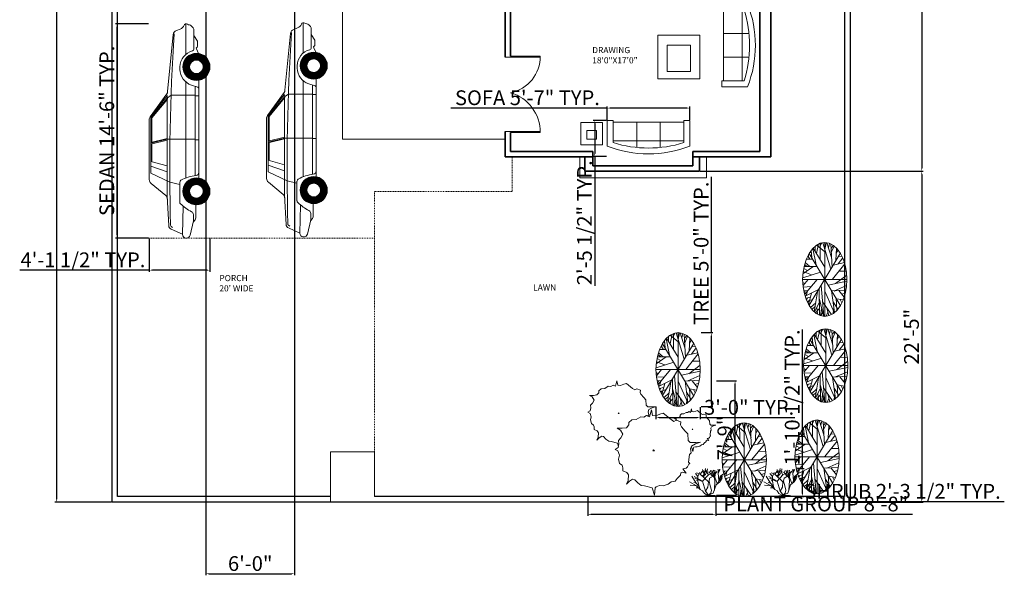
# Model space of a CAD drawing. Units: inches. Extents: x 2562 to 3392, y 1021 to 2243.
# Tile 1 of 6: x 2562 to 3362, y 1021 to 1472. Entities that reach past the tile are written whole.
import ezdxf

# ---------------------------------------------------------------- set-up
doc = ezdxf.new("R2010")
doc.units = ezdxf.units.IN
doc.linetypes.add('JIS_02_0.7', pattern=[1.35, 0.75, -0.6])
for name, color, linetype, lineweight in [('A-ANNO-DIMS', 2, 'Continuous', 18), ('A-ANNO-SYMB', 7, 'Continuous', 13), ('A-AREA-IDEN', 7, 'Continuous', 18), ('A-DOOR', 4, 'Continuous', 18), ('A-FLOR-STRS', 7, 'Continuous', 18), ('A-FURN', 8, 'Continuous', 18), ('A-WALL', 7, 'Continuous', 35), ('C-PKNG-VEHS', 8, 'Continuous', 13), ('C-PROP', 7, 'Continuous', 30), ('L-HRDS', 8, 'Continuous', 18), ('L-HRDS-HIDN', 8, 'JIS_02_0.7', 13), ('L-PLNT', 94, 'Continuous', 13)]:
    doc.layers.add(name, color=color, linetype=linetype, lineweight=lineweight)
doc.styles.get("Standard").update_dxf_attribs({"font": 'arial.ttf'})
doc.dimstyles.new('ISO-25', dxfattribs={"dimtxt": 12, "dimasz": 2.5, "dimexe": 1.25, "dimexo": 0.625, "dimtad": 1, "dimdec": 1, "dimlunit": 3, "dimtxsty": 'Standard', "dimcen": 2.5, "dimadec": 0, "dimazin": 0, "dimtfac": 1, "dimtdec": 1, "dimtmove": 0, "dimatfit": 3, "dimfxl": 1, "dimarcsym": 0})

# ---------------------------------------------------------------- blocks, each defined once
blk = doc.blocks.new('Sofa - Roundback 7 ft.')
for p, q in [((-12.00002, -32.4421), (-12.00003, -6.5971)), ((11.99997, -32.4421), (11.99998, -6.5971)), ((-36.000027, -34), (-36.000027, -11.4696)), ((-35.999844, -13.3819), (35.9998, -13.3819)), ((35.99998, -34), (35.99998, -11.4696)), ((-36.000027, -32.4421), (35.99998, -32.4421))]:
    blk.add_line(p, q)
for points in [[(-36.000027, -34), (-42.000027, -34), (-42.000027, -8)], [(41.99998, -8), (41.99998, -34), (35.99998, -34)]]:
    blk.add_lwpolyline(points)
for centre, radius, start, end in [((0, -114.25), 114.25, 68.43141, 111.5686), ((-0.00001, -127.1968), 121.1968, 72.72033, 107.2797)]:
    blk.add_arc(centre, radius, start, end)
blk = doc.blocks.new('Tree - deciduous plan')
for p, q in [((-32.6092, 50.4264), (-23.2782, 23.5674)), ((-31.2008, 51.1035), (-0.2149, 20.1818)), ((-26.4472, 46.5894), (-26.2712, 53.8116)), ((-22.0458, 42.0753), (-16.5881, 57.6486)), ((-21.1656, 55.8436), (-0.0388, 45.0094)), ((-12.5388, 54.9406), (-7.9613, 59.4546)), ((-12.3627, 32.1443), (-12.5388, 58.7776)), ((-5.3205, 59.6806), (16.5105, 16.7963)), ((2.426, 54.9406), (-1.4472, 59.9056)), ((0, 59.9996), (0, -60)), ((0.4894, 48.6208), (3.6584, 59.6806)), ((18.2711, 35.5298), (5.419, 59.6806)), ((9.8203, 51.5549), (12.8133, 58.5516)), ((19.6795, 19.5047), (16.3344, 57.6486)), ((17.0387, 51.1035), (23.2006, 55.1666)), ((17.7429, 43.6552), (25.4894, 54.2636)), ((31.6513, 50.8778), (30.2429, 30.5643)), ((31.1232, 42.5267), (35.8767, 48.1693)), ((-49.8627, 32.8214), (-32.7853, 32.8214)), ((-45.8134, 38.2383), (-40.5318, 33.0471)), ((-43.8768, 36.4326), (-44.405, 40.2696)), ((42, 42), (-42, -42)), ((42, -42), (-42, 42)), ((-40.1797, 44.558), (-36.4825, 43.2038)), ((-37.0107, 47.0408), (-35.25, 35.5298)), ((36.2288, 25.1474), (48.9049, 35.0784)), ((37.1091, 37.1098), (46.6161, 37.5612)), ((-32.2571, 20.6333), (-59.1937, 9.348)), ((-57.081, 17.9248), (-47.0458, 14.7649)), ((-56.0247, 20.859), (-20.8134, 20.859)), ((-54.7923, 24.4702), (-47.75, 21.0847)), ((-53.2078, 27.4044), (-40.1797, 20.859)), ((54.3626, 25.3731), (20.9119, 0.3198)), ((23.3767, 23.3417), (53.3063, 27.4044)), ((-59.7219, 2.8025), (-12.0106, 12.0565)), ((-58.6656, 12.7336), (-35.9543, 7.5424)), ((-54.6162, -24.7335), (-20.2853, 0.0941)), ((29.3626, -6.6771), (59.4682, 7.091)), ((38.5175, 13.4107), (58.2359, 13.6364)), ((-60, 0), (60, 0)), ((-59.7219, -4.8714), (-54.2641, -6.6771)), ((-45.2853, -0.1316), (-59.0177, -10.0627)), ((-58.4895, -12.3197), (-36.4825, -11.6426)), ((-14.8275, -15.0282), (-14.6515, -57.6865)), ((-10.074, -10.0627), (-2.5036, -59.7178)), ((9.2922, -9.1598), (59.6443, -2.8401)), ((26.3697, -18.4138), (58.9401, -9.8369)), ((-57.081, -18.4138), (-45.2853, -17.9624)), ((-52.6797, -18.188), (-55.4966, -22.0251)), ((-53.2078, -27.442), (-16.7641, -16.6081)), ((-38.9472, -29.0219), (-51.4472, -30.6018)), ((-47.2219, -19.3166), (-50.2148, -26.3135)), ((-46.5177, -30.1504), (-49.5106, -33.536)), ((-35.9543, -22.4765), (-44.0529, -40.5329)), ((-19.9331, -20.2194), (-28.5599, -52.721)), ((-0.0388, -19.0909), (25.8415, -53.8495)), ((18.6232, -18.6394), (26.7218, -53.3981)), ((18.7992, -18.6394), (57.3556, -17.2853)), ((30.419, -30.1504), (32.3556, -50.0125)), ((31.4753, -31.279), (49.6091, -33.3103)), ((38.1654, -18.188), (52.426, -29.0219)), ((45.9119, -24.0564), (55.595, -22.2508)), ((-32.4331, -32.4075), (-48.1021, -35.5674)), ((-43.7008, -34.6645), (-46.6937, -37.373)), ((-24.6867, -37.8244), (-38.7712, -45.7241)), ((-26.2712, -43.9185), (-34.7219, -48.6583)), ((-14.6515, -36.2445), (-27.6797, -52.9467)), ((-14.6515, -47.3041), (-25.0388, -54.3009)), ((-21.5177, -45.4984), (-19.9331, -56.1065)), ((-14.6515, -32.1818), (-3.912, -59.4922)), ((-8.4895, -47.5298), (-11.4825, -58.5893)), ((-6.2008, -36.2445), (17.919, -57.0094)), ((5.9471, -46.6269), (10.5246, -58.5893)), ((22.8485, -36.4702), (35.3485, -48.4326)), ((24.7852, -44.8213), (23.0246, -54.978)), ((41.5105, -32.6332), (46.088, -38.0501)), ((-6.3768, -52.721), (-9.3698, -58.815)), ((8.4119, -53.1724), (3.8344, -59.4922))]:
    blk.add_line(p, q)
blk.add_circle((0, 0), 60)
blk = doc.blocks.new('Shrub - elevation')
for p, q in [((-18.24, 11.04), (-21.755, 16.655)), ((-12.96, 12.48), (-19.68, 16.32)), ((-16.8, 16.32), (-18.72, 18.72)), ((-14.88, 18.24), (-17.76, 19.2)), ((-16.8, 16.32), (-15.36, 19.68)), ((-16.8, 12.48), (-16.8, 16.32)), ((-14.88, 18.24), (-12.96, 20.64)), ((-8.16, 12), (-14.88, 18.24)), ((-13.325, 16.724), (-11.433, 18.289)), ((-12.96, 12.48), (-8.16, 17.76)), ((-12.471, 19.775), (-12.898, 22.044)), ((-11.677, 19.071), (-12.471, 19.775)), ((-11.28, 19.619), (-12.104, 21.184)), ((-12.043, 15.628), (-11.921, 18.836)), ((-11.982, 16.802), (-10.579, 18.054)), ((-11.921, 18.836), (-10.64, 20.401)), ((-11.433, 18.289), (-10.457, 22.749)), ((-10.579, 18.054), (-9.846, 19.697)), ((-8.16, 17.76), (-10.56, 21.6)), ((-9.48, 19.775), (-8.992, 22.592)), ((-7.2, 19.68), (-8.64, 20.16)), ((-8.16, 17.76), (-5.28, 19.2)), ((-7.2, 19.68), (-6.24, 21.12)), ((-4.8, 16.32), (-7.2, 19.68)), ((-7.2, 14.88), (-3.84, 16.8)), ((-5.086, 17.741), (-5.513, 21.34)), ((-5.28, 19.2), (-3.84, 21.6)), ((-3.377, 15.315), (-5.086, 17.819)), ((-2.88, 12.96), (-4.32, 19.68)), ((-3.84, 16.8), (-0.96, 20.64)), ((-3.377, 18.602), (-2.888, 21.575)), ((-2.766, 16.802), (-3.377, 18.602)), ((-2.88, 15.84), (-2.4, 20.16)), ((-0.508, 21.888), (-0.081, 20.558)), ((-0.203, 19.149), (0.102, 21.34)), ((0.346, 13.203), (-0.203, 19.149)), ((-0.142, 19.384), (0.59, 20.401)), ((-0.02, 20.01), (0.896, 21.105)), ((0.041, 20.714), (1.384, 22.044)), ((0.102, 21.34), (0.835, 21.888)), ((0.346, 13.203), (1.323, 16.254)), ((1.323, 16.254), (3.642, 18.289)), ((1.44, 15.36), (2.88, 17.28)), ((2.4, 15.36), (3.36, 16.32)), ((-17.76, 8.64), (-23.663, 11.961)), ((-17.76, 8.64), (-23.128, 9.222)), ((-18.24, 11.04), (-20.16, 11.52)), ((-13.92, 12.48), (-19.2, 14.88)), ((-15.84, 8.16), (-18.24, 11.04)), ((-16.8, 12.48), (-17.76, 12.96)), ((-14.88, 5.76), (-17.76, 8.64)), ((-15.84, 8.16), (-16.8, 12.48)), ((-14.88, 5.76), (-15.84, 8.16)), ((-12.96, 12.48), (-13.92, 12.48)), ((-10.56, 4.32), (-12.96, 12.48)), ((-8.64, 7.68), (-8.16, 12)), ((-7.68, 12.48), (-7.2, 14.88)), ((-6.72, 8.64), (-7.68, 12.48)), ((-5.76, 5.28), (-6.72, 8.64)), ((-4.32, 2.88), (-1.92, 9.6)), ((-3.36, 5.28), (-2.88, 12.96)), ((-0.96, 10.56), (-2.88, 15.84)), ((-1.92, 9.6), (0.96, 12)), ((-0.48, 10.8), (0.346, 13.203)), ((0.96, 12), (1.44, 15.36)), ((0.96, 12), (2.88, 14.88)), ((1.92, 13.44), (2.4, 15.36)), ((-16.32, 7.2), (-18.24, 7.2)), ((-15.84, 0.48), (-17.76, 0)), ((-13.44, 0.48), (-15.84, 0.48)), ((-12.96, 4.8), (-14.88, 5.76)), ((-9.6, 0.96), (-13.44, 0.48)), ((-11.52, 2.4), (-12.96, 4.8)), ((-9.6, 0.96), (-12.96, 0)), ((-8.64, 0.96), (-11.52, 2.4)), ((-10.56, 4.32), (-8.64, 7.68)), ((-8.64, 1.92), (-10.56, 4.32)), ((-9.6, 0.96), (-7.68, 0.96)), ((-8.64, 0.96), (-4.32, 2.88)), ((-8.64, 0.96), (-6.24, 2.88)), ((-8.64, 0.96), (-8.64, 1.92)), ((-8.64, 0.96), (-2.88, 0.96)), ((-7.68, 0.96), (-6.24, 0.48)), ((-6.24, 2.88), (-5.76, 5.28)), ((-6.24, 0.48), (-3.36, 0)), ((-2.88, 0.96), (0, 0))]:
    blk.add_line(p, q)
blk = doc.blocks.new('Clump of Trees or Bushes - plan')
for points in [[(-10.993, 56.487), (-9.228, 58.426), (-10.144, 63.512), (-8.923, 67.033), (-3.43, 69.772), (2.673, 72.119), (-2.82, 71.728), (-10.449, 71.728), (-13.195, 74.075), (-13.806, 83.073), (-16.857, 86.594), (-22.045, 92.071), (-22.961, 94.81), (-22.656, 98.722), (-28.759, 100.678), (-31.811, 99.113), (-35.472, 101.461), (-45.543, 109.676), (-49.815, 108.503), (-55.308, 106.155), (-59.58, 106.938), (-60.801, 113.98), (-63.242, 104.982), (-67.209, 106.938), (-70.872, 104.59), (-74.839, 104.982), (-80.637, 101.461), (-86.435, 101.069), (-90.402, 97.548), (-90.402, 94.419), (-93.454, 90.898), (-98.947, 90.115), (-105.66, 90.115), (-101.083, 87.768), (-98.031, 82.682), (-100.778, 77.596), (-103.829, 74.466), (-103.219, 69.772), (-104.134, 65.077), (-108.102, 62.73), (-104.439, 60.774), (-102.609, 55.297), (-103.829, 50.211), (-102.303, 44.342), (-98.947, 41.995), (-98.031, 38.865), (-98.031, 34.953), (-93.148, 32.606), (-90.707, 29.476), (-91.317, 22.434), (-93.454, 17.348), (-89.487, 21.26), (-85.519, 23.999), (-82.468, 23.216), (-78.806, 19.304), (-74.228, 15.783), (-69.956, 15.392), (-59.886, 12.653), (-58.254, 7.074)], [(59.448, 5.262), (60.936, 4.858), (62.652, -1.011), (63.415, 4.858), (64.178, 5.836), (66.848, 6.814), (69.709, 6.569), (73.905, 7.792), (76.385, 9.748), (79.627, 10.237), (81.153, 12.438), (84.014, 15.127), (84.205, 17.084), (85.158, 17.573), (88.591, 16.839), (85.73, 20.262), (88.591, 20.751), (89.545, 21.974), (90.689, 24.174), (91.452, 24.663), (90.499, 25.886), (91.261, 31.999), (92.596, 33.466), (92.024, 36.645), (92.787, 38.845), (96.22, 40.557), (100.035, 42.024), (96.602, 41.779), (91.834, 41.779), (90.117, 43.246), (89.736, 48.871), (87.828, 51.071), (84.586, 54.494), (84.014, 56.206), (84.205, 58.651), (80.39, 59.873), (78.483, 58.895), (76.194, 60.362), (69.9, 65.497), (67.23, 64.764), (63.797, 63.297), (61.126, 63.786), (60.364, 68.187), (58.838, 62.563), (56.358, 63.786), (54.07, 62.319), (51.59, 62.563), (47.966, 60.362), (44.343, 60.118), (41.863, 57.917), (41.863, 55.961), (39.956, 53.761), (36.523, 53.272), (32.327, 53.272), (35.187, 51.805), (36.641, 49.381)]]:
    blk.add_lwpolyline(points)
for points in [[(-4.577, 66.508), (-7.629, 55.261), (-12.588, 57.706), (-17.166, 54.772), (-22.125, 55.261), (-29.372, 50.86), (-36.62, 50.371), (-41.579, 45.969), (-41.579, 42.057), (-45.393, 37.656), (-52.259, 36.678), (-60.651, 36.678), (-54.93, 33.743), (-51.115, 27.386), (-54.548, 21.029), (-58.363, 17.116), (-57.6, 11.248), (-58.744, 5.38), (-63.703, 2.446), (-59.126, 0), (-56.837, -6.846), (-58.363, -13.203), (-56.455, -20.539), (-52.259, -23.473), (-51.115, -27.385), (-51.115, -32.275), (-45.012, -35.21), (-41.96, -39.122), (-42.723, -47.924), (-45.393, -54.282), (-40.434, -49.391), (-35.475, -45.968), (-31.661, -46.946), (-27.083, -51.837), (-21.362, -56.238), (-16.021, -56.727), (-3.433, -60.15), (0, -71.887), (1.526, -60.15), (3.052, -58.194), (8.392, -56.238), (14.114, -56.727), (22.506, -54.282), (27.465, -50.369), (33.949, -49.391), (37.001, -44.99), (42.723, -39.611), (43.104, -35.699), (45.012, -34.721), (51.878, -36.188), (46.156, -29.341), (51.878, -28.363), (53.785, -25.918), (56.074, -21.517), (57.6, -20.539), (55.692, -18.094), (57.218, -5.868), (59.888, -2.934), (58.744, 3.424), (60.27, 7.825), (67.136, 11.248), (74.765, 14.182), (67.899, 13.693), (58.363, 13.693), (54.93, 16.627), (54.167, 27.875), (50.352, 32.276), (43.867, 39.123), (42.723, 42.546), (43.104, 47.436), (35.475, 49.882), (31.661, 47.925), (27.083, 50.86), (14.495, 61.129), (9.155, 59.662), (2.289, 56.728), (-3.052, 57.706)], [(-58.055, 61.947), (-58.97, 60.774), (-57.139, 60.774)], [(62.08, 35.667), (61.508, 34.933), (62.652, 34.933)], [(-1.144, 1.468), (-2.289, 0), (0, 0)]]:
    blk.add_lwpolyline(points, close=True)
blk = doc.blocks.new('Seam Weld')
for p, q in [((-0.2, -0.099999), (0.2, -0.099999)), ((0.2, -0.2), (-0.2, -0.2))]:
    blk.add_line(p, q)
blk.add_circle((0, -0.15), 0.15)
blk = doc.blocks.new('Car - sedan  side')
for p, q in [((-77.81, 49.34), (-126.58, 49.34)), ((-56.87, 35.13), (-75.48, 48.59)), ((-139.53, 35.99), (-129.64, 47.91)), ((-128.57, 32.64), (-121.22, 48.02)), ((-74.7, 48.02), (-121.22, 48.02)), ((-120.32, 34.67), (-115.67, 48.02)), ((-115.4, 34.67), (-111.74, 48.02)), ((-97.55, 47.3), (-111.94, 47.3)), ((-94.41, 34.67), (-97.73, 48.02)), ((-93.72, 34.67), (-97.04, 48.02)), ((-93.03, 34.67), (-96.34, 48.02)), ((-76.26, 47.3), (-96.16, 47.3)), ((-61.08, 34.66), (-76.26, 47.3)), ((-60.02, 34.65), (-76.07, 48.02)), ((-58.54, 34.93), (-74.99, 48.02)), ((-140.23, 34.67), (-163.88, 33.56)), ((-62.28, 34.67), (-140.23, 34.67)), ((-130.39, 24.63), (-128.57, 32.64)), ((-93.72, 19.62), (-93.72, 34.67)), ((-62.28, 34.67), (-60.02, 34.65)), ((-60.02, 34.65), (-58.54, 34.93)), ((-57.97, 31.61), (-60.02, 34.65)), ((-57.21, 35.38), (-58.54, 34.93)), ((-54.93, 34.4), (-8.75, 29.8)), ((-170.93, 22.32), (-166.81, 31.56)), ((-164.57, 31.6), (-165.48, 30.35)), ((-128.78, 24.63), (-144.79, 24.63)), ((-57.97, 19.62), (-57.97, 31.61)), ((-36.97, 24.38), (-34.94, 24.38)), ((-4.21, 24.18), (-5.42, 27.27)), ((-174, 19.51), (-174, 18.91)), ((-160.12, 13.48), (-171.81, 16.16)), ((-148.26, 21.7), (-171.11, 22.33)), ((-47.2, 19.62), (-125.23, 19.62)), ((-93.72, 12.14), (-93.72, 19.62)), ((-57.97, 12.14), (-57.97, 19.62)), ((0, 19.62), (-24.7, 19.62)), ((-159.22, 12.14), (-161.08, 13.7)), ((-155.01, 13.48), (-160.12, 13.48)), ((-147.03, 11.6), (-157.73, 11.6)), ((-120.62, 9.03), (-125.23, 9.03)), ((-50.67, 12.14), (-123.32, 12.14)), ((-45.76, 9.03), (-120.62, 9.03)), ((-94.21, 9.03), (-94.21, 12.14)), ((-58.39, 9.03), (-58.39, 12.14)), ((-51.4, 9.89), (-49.69, 15.14)), ((-20.36, 11.06), (-24.06, 9.44)), ((-4.23, 13.19), (-20.72, 13.19)), ((-18.83, 10.42), (-19.11, 10.76)), ((-14.68, 10.03), (-18.01, 10.03)), ((-9.5, 13.19), (-14.1, 10.2)), ((-3.22, 13.59), (-1.77, 14.97))]:
    blk.add_line(p, q)
at = {"const_width": 5.49}
for points in [[(-127.8, 11, -1), (-144.3, 11, -1)], [(-26.69, 11, -1), (-43.19, 11, -1)]]:
    blk.add_lwpolyline(points, format="xyb", close=True, dxfattribs=at)
for centre, radius in [((-136.05, 11), 11), ((-136.05, 11), 5.51), ((-34.94, 11), 11), ((-34.94, 11), 5.51)]:
    blk.add_circle(centre, radius)
for centre, radius, start, end in [((-126.58, 45.38), 3.97, 90, 140.30288), ((-77.81, 45.38), 3.97, 54.13504, 90), ((-163.72, 30.18), 3.38, 92.68266, 155.97362), ((-163.62, 30.91), 1.17, 91.49105, 143.95527), ((-118.51, -1702.12), 1734.79, 86.34698, 91.49105), ((-142.58, 38.53), 3.97, 272.68265, 320.30288), ((-54.54, 38.35), 3.97, 234.13503, 264.31231), ((-144.79, 22.64), 1.98, 90, 136.3964), ((-128.78, 22.64), 1.98, 28.1371, 90), ((-36.97, 11), 13.38, 90, 161.97316), ((-34.94, 11), 13.38, 13.58642, 90), ((-9.15, 25.82), 4, 21.31069, 84.3123), ((0.9, 26.18), 5.49, 201.3107, 247.70484), ((-171.18, 19.51), 2.82, 88.41927, 180), ((-171.18, 18.91), 2.82, 180, 257.09053), ((-118.09, -2.78), 38.85, 136.3964, 152.90974), ((-157.14, 7.48), 34.14, 6.51354, 28.1371), ((-3.82, 17.12), 2.96, 313.71735, 352.38387), ((-1.92, 19.3), 1.94, 325.37436, 67.70485), ((2.46, 16.28), 3.37, 145.37437, 172.38386), ((-157.73, 13.93), 2.32, 230.12913, 270), ((-155.01, 16.1), 2.62, 270, 332.90974), ((-120.62, 11.65), 2.62, 186.51353, 270), ((-52.58, 10.27), 1.24, 270, 341.97316), ((-20.72, 14.43), 1.24, 193.58641, 270), ((-19.93, 10.09), 1.06, 39.30103, 113.71592), ((-18.01, 11.09), 1.06, 219.30104, 270), ((-14.68, 11.09), 1.06, 270, 303.04697), ((-4.23, 14.65), 1.46, 270, 313.71735)]:
    blk.add_arc(centre, radius, start, end)
blk = doc.blocks.new('*D22')
at = {"layer": 'A-ANNO-DIMS', "color": 0, "lineweight": -2, "transparency": 16777216}
for p, q in [((2636.14, 2160.13), (2590.2, 2160.13)), ((2591.45, 2157.63), (2591.45, 1082.63)), ((2636.14, 1080.13), (2590.2, 1080.13))]:
    blk.add_line(p, q, dxfattribs=at)
at = {"layer": 'A-ANNO-DIMS', "color": 0, "transparency": 16777216}
for points in [[(2591.03, 2157.63), (2591.86, 2157.63), (2591.45, 2160.13)], [(2591.03, 1082.63), (2591.86, 1082.63), (2591.45, 1080.13)]]:
    blk.add_solid(points, dxfattribs=at)
at = {"layer": 'Defpoints', "color": 0, "transparency": 16777216}
for p in [(2636.76, 2160.13), (2591.45, 1080.13), (2636.76, 1080.13)]:
    blk.add_point(p, dxfattribs=at)
at = {"layer": 'A-ANNO-DIMS', "color": 0, "transparency": 16777216, "insert": (2584.7, 1620.13), "char_height": 12, "attachment_point": 5, "rotation": 90}
blk.add_mtext("90'", dxfattribs=at)
blk = doc.blocks.new('*D39')
at = {"layer": 'A-ANNO-DIMS', "color": 0, "lineweight": -2, "transparency": 16777216}
for p, q in [((3039.22, 1390.89), (3039.22, 1401.59)), ((3106.42, 1390.89), (3106.42, 1401.59)), ((3039.22, 1400.34), (2912.08, 1400.34)), ((3103.92, 1400.34), (3041.72, 1400.34))]:
    blk.add_line(p, q, dxfattribs=at)
at = {"layer": 'A-ANNO-DIMS', "color": 0, "transparency": 16777216}
for points in [[(3041.72, 1400.76), (3041.72, 1399.92), (3039.22, 1400.34)], [(3103.92, 1400.76), (3103.92, 1399.92), (3106.42, 1400.34)]]:
    blk.add_solid(points, dxfattribs=at)
at = {"layer": 'Defpoints', "color": 0, "transparency": 16777216}
for p in [(3039.22, 1400.34), (3039.22, 1390.26), (3106.42, 1390.26)]:
    blk.add_point(p, dxfattribs=at)
at = {"layer": 'A-ANNO-DIMS', "color": 0, "transparency": 16777216, "insert": (2974.4, 1407.17), "char_height": 12, "attachment_point": 5}
blk.add_mtext('SOFA 5\'-7" TYP.', dxfattribs=at)
blk = doc.blocks.new('*D40')
at = {"layer": 'A-ANNO-DIMS', "color": 0, "lineweight": -2, "transparency": 16777216}
for p, q in [((3038.6, 1390.26), (3027.89, 1390.26)), ((3029.14, 1387.76), (3029.14, 1363.43)), ((3038.6, 1360.93), (3027.89, 1360.93)), ((3029.14, 1360.93), (3029.14, 1255.86))]:
    blk.add_line(p, q, dxfattribs=at)
at = {"layer": 'A-ANNO-DIMS', "color": 0, "transparency": 16777216}
for points in [[(3028.73, 1387.76), (3029.56, 1387.76), (3029.14, 1390.26)], [(3028.73, 1363.43), (3029.56, 1363.43), (3029.14, 1360.93)]]:
    blk.add_solid(points, dxfattribs=at)
at = {"layer": 'Defpoints', "color": 0, "transparency": 16777216}
for p in [(3039.22, 1390.26), (3029.14, 1360.93), (3039.22, 1360.93)]:
    blk.add_point(p, dxfattribs=at)
at = {"layer": 'A-ANNO-DIMS', "color": 0, "transparency": 16777216, "insert": (3022.31, 1307.15), "char_height": 12, "attachment_point": 5, "rotation": 90}
blk.add_mtext('2\'-5 1/2" TYP.', dxfattribs=at)
blk = doc.blocks.new('*D43')
at = {"layer": 'A-ANNO-DIMS', "color": 0, "lineweight": -2, "transparency": 16777216}
for p, q in [((3016.09, 1486), (3016.09, 1481.77)), ((3018.59, 1483.02), (3037.59, 1483.02)), ((3040.09, 1486), (3040.09, 1481.77)), ((3040.09, 1483.02), (3214.18, 1483.02))]:
    blk.add_line(p, q, dxfattribs=at)
at = {"layer": 'A-ANNO-DIMS', "color": 0, "transparency": 16777216}
for points in [[(3018.59, 1483.44), (3018.59, 1482.6), (3016.09, 1483.02)], [(3037.59, 1483.44), (3037.59, 1482.6), (3040.09, 1483.02)]]:
    blk.add_solid(points, dxfattribs=at)
at = {"layer": 'Defpoints', "color": 0, "transparency": 16777216}
for p in [(3016.09, 1486.62), (3040.09, 1486.62), (3040.09, 1483.02)]:
    blk.add_point(p, dxfattribs=at)
at = {"layer": 'A-ANNO-DIMS', "color": 0, "transparency": 16777216, "insert": (3128.38, 1489.77), "char_height": 12, "attachment_point": 5}
blk.add_mtext('END TABLE 2\'-0" TYP.', dxfattribs=at)
blk = doc.blocks.new('*D49')
at = {"layer": 'A-ANNO-DIMS', "color": 0, "lineweight": -2, "transparency": 16777216}
for p, q in [((2666.35, 1468.87), (2639.61, 1468.87)), ((2640.86, 1297.25), (2640.86, 1466.37)), ((2666.35, 1294.75), (2639.61, 1294.75))]:
    blk.add_line(p, q, dxfattribs=at)
at = {"layer": 'A-ANNO-DIMS', "color": 0, "transparency": 16777216}
for points in [[(2640.44, 1466.37), (2641.27, 1466.37), (2640.86, 1468.87)], [(2640.44, 1297.25), (2641.27, 1297.25), (2640.86, 1294.75)]]:
    blk.add_solid(points, dxfattribs=at)
at = {"layer": 'Defpoints', "color": 0, "transparency": 16777216}
for p in [(2640.86, 1468.87), (2666.97, 1468.87), (2666.97, 1294.75)]:
    blk.add_point(p, dxfattribs=at)
at = {"layer": 'A-ANNO-DIMS', "color": 0, "transparency": 16777216, "insert": (2634.03, 1381.81), "char_height": 12, "attachment_point": 5, "rotation": 90}
blk.add_mtext('SEDAN 14\'-6" TYP.', dxfattribs=at)
blk = doc.blocks.new('*D50')
at = {"layer": 'A-ANNO-DIMS', "color": 0, "lineweight": -2, "transparency": 16777216}
for p, q in [((2666.97, 1294.13), (2666.97, 1267.39)), ((2716.32, 1294.13), (2716.32, 1267.39)), ((2666.97, 1268.64), (2561.63, 1268.64)), ((2713.82, 1268.64), (2669.47, 1268.64))]:
    blk.add_line(p, q, dxfattribs=at)
at = {"layer": 'A-ANNO-DIMS', "color": 0, "transparency": 16777216}
for points in [[(2669.47, 1269.05), (2669.47, 1268.22), (2666.97, 1268.64)], [(2713.82, 1269.05), (2713.82, 1268.22), (2716.32, 1268.64)]]:
    blk.add_solid(points, dxfattribs=at)
at = {"layer": 'Defpoints', "color": 0, "transparency": 16777216}
for p in [(2666.97, 1294.75), (2716.32, 1294.75), (2666.97, 1268.64)]:
    blk.add_point(p, dxfattribs=at)
at = {"layer": 'A-ANNO-DIMS', "color": 0, "transparency": 16777216, "insert": (2613.05, 1275.47), "char_height": 12, "attachment_point": 5}
blk.add_mtext('4\'-1 1/2" TYP.', dxfattribs=at)
blk = doc.blocks.new('*D51')
at = {"layer": 'A-ANNO-DIMS', "color": 0, "lineweight": -2, "transparency": 16777216}
for p, q in [((3123.92, 1217.84), (3123.92, 1344.41)), ((3115.55, 1217.84), (3125.17, 1217.84)), ((3123.92, 1160.34), (3123.92, 1215.34)), ((3115.55, 1157.84), (3125.17, 1157.84))]:
    blk.add_line(p, q, dxfattribs=at)
at = {"layer": 'A-ANNO-DIMS', "color": 0, "transparency": 16777216}
for points in [[(3123.51, 1215.34), (3124.34, 1215.34), (3123.92, 1217.84)], [(3123.51, 1160.34), (3124.34, 1160.34), (3123.92, 1157.84)]]:
    blk.add_solid(points, dxfattribs=at)
at = {"layer": 'Defpoints', "color": 0, "transparency": 16777216}
for p in [(3114.92, 1217.84), (3123.92, 1217.84), (3114.92, 1157.84)]:
    blk.add_point(p, dxfattribs=at)
at = {"layer": 'A-ANNO-DIMS', "color": 0, "transparency": 16777216, "insert": (3117.17, 1282.37), "char_height": 12, "attachment_point": 5, "rotation": 90}
blk.add_mtext('TREE 5\'-0" TYP.', dxfattribs=at)
blk = doc.blocks.new('*D52')
at = {"layer": 'A-ANNO-DIMS', "color": 0, "lineweight": -2, "transparency": 16777216}
for p, q in [((3078.92, 1157.22), (3078.92, 1147.59)), ((3114.92, 1157.22), (3114.92, 1147.59)), ((3081.42, 1148.84), (3112.42, 1148.84)), ((3114.92, 1148.84), (3191.81, 1148.84))]:
    blk.add_line(p, q, dxfattribs=at)
at = {"layer": 'A-ANNO-DIMS', "color": 0, "transparency": 16777216}
for points in [[(3081.42, 1149.26), (3081.42, 1148.42), (3078.92, 1148.84)], [(3112.42, 1149.26), (3112.42, 1148.42), (3114.92, 1148.84)]]:
    blk.add_solid(points, dxfattribs=at)
at = {"layer": 'Defpoints', "color": 0, "transparency": 16777216}
for p in [(3078.92, 1157.84), (3114.92, 1157.84), (3114.92, 1148.84)]:
    blk.add_point(p, dxfattribs=at)
at = {"layer": 'A-ANNO-DIMS', "color": 0, "transparency": 16777216, "insert": (3154.62, 1155.6), "char_height": 12, "attachment_point": 5}
blk.add_mtext('3\'-0" TYP.', dxfattribs=at)
blk = doc.blocks.new('*D57')
at = {"layer": 'A-ANNO-DIMS', "color": 0, "lineweight": -2, "transparency": 16777216}
for p, q in [((3166.64, 1084.01), (3166.64, 1079.29)), ((3193.94, 1084.01), (3193.94, 1079.29)), ((3169.14, 1080.54), (3191.44, 1080.54)), ((3193.94, 1080.54), (3362.08, 1080.54))]:
    blk.add_line(p, q, dxfattribs=at)
at = {"layer": 'A-ANNO-DIMS', "color": 0, "transparency": 16777216}
for points in [[(3169.14, 1080.95), (3169.14, 1080.12), (3166.64, 1080.54)], [(3191.44, 1080.95), (3191.44, 1080.12), (3193.94, 1080.54)]]:
    blk.add_solid(points, dxfattribs=at)
at = {"layer": 'Defpoints', "color": 0, "transparency": 16777216}
for p in [(3166.64, 1084.63), (3193.94, 1084.63), (3193.94, 1080.54)]:
    blk.add_point(p, dxfattribs=at)
at = {"layer": 'A-ANNO-DIMS', "color": 0, "transparency": 16777216, "insert": (3279.26, 1087.37), "char_height": 12, "attachment_point": 5}
blk.add_mtext('SHRUB 2\'-3 1/2" TYP.', dxfattribs=at)
blk = doc.blocks.new('*D58')
at = {"layer": 'A-ANNO-DIMS', "color": 0, "lineweight": -2, "transparency": 16777216}
for p, q in [((3198.04, 1107.38), (3198.04, 1220.43)), ((3194.57, 1107.38), (3199.29, 1107.38)), ((3198.04, 1087.13), (3198.04, 1104.88)), ((3194.57, 1084.63), (3199.29, 1084.63))]:
    blk.add_line(p, q, dxfattribs=at)
at = {"layer": 'A-ANNO-DIMS', "color": 0, "transparency": 16777216}
for points in [[(3197.62, 1104.88), (3198.46, 1104.88), (3198.04, 1107.38)], [(3197.62, 1087.13), (3198.46, 1087.13), (3198.04, 1084.63)]]:
    blk.add_solid(points, dxfattribs=at)
at = {"layer": 'Defpoints', "color": 0, "transparency": 16777216}
for p in [(3193.94, 1107.38), (3198.04, 1107.38), (3193.94, 1084.63)]:
    blk.add_point(p, dxfattribs=at)
at = {"layer": 'A-ANNO-DIMS', "color": 0, "transparency": 16777216, "insert": (3191.21, 1165.16), "char_height": 12, "attachment_point": 5, "rotation": 90}
blk.add_mtext('1\'-10 1/2" TYP.', dxfattribs=at)
blk = doc.blocks.new('*D59')
at = {"layer": 'A-ANNO-DIMS', "color": 0, "lineweight": -2, "transparency": 16777216}
for p, q in [((2753.12, 1494.79), (2753.12, 1497.46)), ((2766.77, 1494.79), (2766.77, 1497.46)), ((2755.62, 1496.21), (2764.27, 1496.21)), ((2766.77, 1496.21), (2934.91, 1496.21))]:
    blk.add_line(p, q, dxfattribs=at)
at = {"layer": 'A-ANNO-DIMS', "color": 0, "transparency": 16777216}
for points in [[(2755.62, 1496.63), (2755.62, 1495.8), (2753.12, 1496.21)], [(2764.27, 1496.63), (2764.27, 1495.8), (2766.77, 1496.21)]]:
    blk.add_solid(points, dxfattribs=at)
at = {"layer": 'Defpoints', "color": 0, "transparency": 16777216}
for p in [(2753.12, 1494.16), (2766.77, 1496.21), (2766.77, 1494.16)]:
    blk.add_point(p, dxfattribs=at)
at = {"layer": 'A-ANNO-DIMS', "color": 0, "transparency": 16777216, "insert": (2852.09, 1503.04), "char_height": 12, "attachment_point": 5}
blk.add_mtext('SHRUB 1\'-1 1/2" TYP.', dxfattribs=at)
blk = doc.blocks.new('*D61')
at = {"layer": 'A-ANNO-DIMS', "color": 0, "lineweight": -2, "transparency": 16777216}
for p, q in [((3023.54, 1085.21), (3023.54, 1068.98)), ((3127.6, 1085.21), (3127.6, 1068.98)), ((3026.04, 1070.23), (3125.1, 1070.23)), ((3127.6, 1070.23), (3287.48, 1070.23))]:
    blk.add_line(p, q, dxfattribs=at)
at = {"layer": 'A-ANNO-DIMS', "color": 0, "transparency": 16777216}
for points in [[(3026.04, 1070.64), (3026.04, 1069.81), (3023.54, 1070.23)], [(3125.1, 1070.64), (3125.1, 1069.81), (3127.6, 1070.23)]]:
    blk.add_solid(points, dxfattribs=at)
at = {"layer": 'Defpoints', "color": 0, "transparency": 16777216}
for p in [(3023.54, 1085.84), (3127.6, 1085.84), (3127.6, 1070.23)]:
    blk.add_point(p, dxfattribs=at)
at = {"layer": 'A-ANNO-DIMS', "color": 0, "transparency": 16777216, "insert": (3208.79, 1077.06), "char_height": 12, "attachment_point": 5}
blk.add_mtext('PLANT GROUP 8\'-8"', dxfattribs=at)
blk = doc.blocks.new('*D62')
at = {"layer": 'A-ANNO-DIMS', "color": 0, "lineweight": -2, "transparency": 16777216}
for p, q in [((3128.23, 1178.77), (3144.46, 1178.77)), ((3143.21, 1088.34), (3143.21, 1176.27)), ((3128.23, 1085.84), (3144.46, 1085.84))]:
    blk.add_line(p, q, dxfattribs=at)
at = {"layer": 'A-ANNO-DIMS', "color": 0, "transparency": 16777216}
for points in [[(3142.8, 1176.27), (3143.63, 1176.27), (3143.21, 1178.77)], [(3142.8, 1088.34), (3143.63, 1088.34), (3143.21, 1085.84)]]:
    blk.add_solid(points, dxfattribs=at)
at = {"layer": 'Defpoints', "color": 0, "transparency": 16777216}
for p in [(3127.6, 1178.77), (3143.21, 1178.77), (3127.6, 1085.84)]:
    blk.add_point(p, dxfattribs=at)
at = {"layer": 'A-ANNO-DIMS', "color": 0, "transparency": 16777216, "insert": (3136.46, 1132.3), "char_height": 12, "attachment_point": 5, "rotation": 90}
blk.add_mtext('7\'-9"', dxfattribs=at)
blk = doc.blocks.new('*D67')
at = {"layer": 'A-ANNO-DIMS', "color": 0, "lineweight": -2, "transparency": 16777216}
for p, q in [((2712.95, 1482.01), (2712.95, 1478.58)), ((2731.65, 1482.01), (2731.65, 1478.58)), ((2715.45, 1479.83), (2729.15, 1479.83)), ((2731.65, 1479.83), (2894.6, 1479.83))]:
    blk.add_line(p, q, dxfattribs=at)
at = {"layer": 'A-ANNO-DIMS', "color": 0, "transparency": 16777216}
for points in [[(2715.45, 1480.24), (2715.45, 1479.41), (2712.95, 1479.83)], [(2729.15, 1480.24), (2729.15, 1479.41), (2731.65, 1479.83)]]:
    blk.add_solid(points, dxfattribs=at)
at = {"layer": 'Defpoints', "color": 0, "transparency": 16777216}
for p in [(2712.95, 1482.63), (2731.65, 1482.63), (2731.65, 1479.83)]:
    blk.add_point(p, dxfattribs=at)
at = {"layer": 'A-ANNO-DIMS', "color": 0, "transparency": 16777216, "insert": (2814.37, 1486.66), "char_height": 12, "attachment_point": 5}
blk.add_mtext('PLANT 1\'-6 1/2" TYP.', dxfattribs=at)
blk = doc.blocks.new('*D70')
at = {"layer": 'A-ANNO-DIMS', "color": 0, "lineweight": -2, "transparency": 16777216}
for p, q in [((3172.89, 2095.63), (3296.21, 2095.63)), ((3294.96, 2093.13), (3294.96, 1351.49)), ((3114.84, 1348.99), (3296.21, 1348.99))]:
    blk.add_line(p, q, dxfattribs=at)
at = {"layer": 'A-ANNO-DIMS', "color": 0, "transparency": 16777216}
for points in [[(3294.55, 2093.13), (3295.38, 2093.13), (3294.96, 2095.63)], [(3294.55, 1351.49), (3295.38, 1351.49), (3294.96, 1348.99)]]:
    blk.add_solid(points, dxfattribs=at)
at = {"layer": 'Defpoints', "color": 0, "transparency": 16777216}
for p in [(3172.26, 2095.63), (3114.22, 1348.99), (3294.96, 1348.99)]:
    blk.add_point(p, dxfattribs=at)
at = {"layer": 'A-ANNO-DIMS', "color": 0, "transparency": 16777216, "insert": (3288.13, 1722.31), "char_height": 12, "attachment_point": 5, "rotation": 90}
blk.add_mtext('62\'-2 1/2"', dxfattribs=at)
blk = doc.blocks.new('*D73')
at = {"layer": 'A-ANNO-DIMS', "color": 0, "lineweight": -2, "transparency": 16777216}
for p, q in [((3114.84, 1348.99), (3296.21, 1348.99)), ((3294.96, 1346.49), (3294.96, 1082.63)), ((3237.39, 1080.13), (3296.21, 1080.13))]:
    blk.add_line(p, q, dxfattribs=at)
at = {"layer": 'A-ANNO-DIMS', "color": 0, "transparency": 16777216}
for points in [[(3294.55, 1346.49), (3295.38, 1346.49), (3294.96, 1348.99)], [(3294.55, 1082.63), (3295.38, 1082.63), (3294.96, 1080.13)]]:
    blk.add_solid(points, dxfattribs=at)
at = {"layer": 'Defpoints', "color": 0, "transparency": 16777216}
for p in [(3114.22, 1348.99), (3236.76, 1080.13), (3294.96, 1080.13)]:
    blk.add_point(p, dxfattribs=at)
at = {"layer": 'A-ANNO-DIMS', "color": 0, "transparency": 16777216, "insert": (3288.21, 1214.56), "char_height": 12, "attachment_point": 5, "rotation": 90}
blk.add_mtext('22\'-5"', dxfattribs=at)
blk = doc.blocks.new('*D78')
at = {"layer": 'A-ANNO-DIMS', "color": 0, "lineweight": -2, "transparency": 16777216}
for p, q in [((2712.95, 1482.01), (2712.95, 1020.68)), ((2785.11, 1482.01), (2785.11, 1020.68)), ((2715.45, 1021.93), (2782.61, 1021.93))]:
    blk.add_line(p, q, dxfattribs=at)
at = {"layer": 'A-ANNO-DIMS', "color": 0, "transparency": 16777216}
for points in [[(2715.45, 1022.35), (2715.45, 1021.52), (2712.95, 1021.93)], [(2782.61, 1022.35), (2782.61, 1021.52), (2785.11, 1021.93)]]:
    blk.add_solid(points, dxfattribs=at)
at = {"layer": 'Defpoints', "color": 0, "transparency": 16777216}
for p in [(2712.95, 1482.63), (2785.11, 1482.63), (2785.11, 1021.93)]:
    blk.add_point(p, dxfattribs=at)
at = {"layer": 'A-ANNO-DIMS', "color": 0, "transparency": 16777216, "insert": (2749.03, 1028.68), "char_height": 12, "attachment_point": 5}
blk.add_mtext('6\'-0"', dxfattribs=at)

msp = doc.modelspace()

# ---------------------------------------------------------------- linework, layer by layer
at = {"layer": 'A-DOOR'}
for p, q in [((2956.26, 1441.58), (2960.76, 1441.58)), ((2984.76, 1442.58), (2960.76, 1442.58)), ((2960.76, 1441.58), (2984.76, 1441.58)), ((2984.76, 1441.58), (2984.76, 1442.58)), ((2984.76, 1381.42), (2956.26, 1381.42)), ((2960.76, 1380.42), (2984.76, 1380.42)), ((2984.76, 1380.42), (2984.76, 1381.42))]:
    msp.add_line(p, q, dxfattribs=at)
for centre, radius, start, end in [((2954.83, 1442.08), 29.94, 281.43599, 0.95687), ((2951.67, 1380.92), 33.09, 359.13428, 74.05898)]:
    msp.add_arc(centre, radius, start, end, dxfattribs=at)
at = {"layer": 'A-FLOR-STRS'}
for p, q in [((3016.87, 1343.69), (3016.87, 1360.63)), ((3119.87, 1360.63), (3119.87, 1343.69)), ((3119.87, 1343.69), (3016.87, 1343.69))]:
    msp.add_line(p, q, dxfattribs=at)
at = {"layer": 'A-FURN'}
for points in [[(3080.37, 1459.59), (3114.63, 1459.59), (3114.63, 1424.17), (3080.37, 1424.17)], [(3087.99, 1451.42), (3106.88, 1451.42), (3106.88, 1429.94), (3087.99, 1429.94)], [(3017.74, 1388.49), (3035.53, 1388.49), (3035.53, 1370.53), (3017.74, 1370.53)], [(3022.79, 1382), (3030.61, 1382), (3030.61, 1374.98), (3022.79, 1374.98)]]:
    msp.add_lwpolyline(points, close=True, dxfattribs=at)
at = {"layer": 'A-WALL'}
for p, q in [((3172.26, 2095.63), (3172.26, 1360.63)), ((3163.26, 2086.63), (3163.26, 1365.13)), ((2960.76, 1510.44), (2960.76, 1442.58)), ((2956.26, 1500.7), (2956.26, 1441.58)), ((2956.26, 1381.42), (2956.26, 1360.63)), ((2960.76, 1380.42), (2960.76, 1365.13)), ((2960.76, 1365.13), (3027.7, 1365.13)), ((3027.7, 1365.13), (3027.7, 1353.4)), ((3108.88, 1353.4), (3108.88, 1365.13)), ((3108.88, 1365.13), (3163.26, 1365.13)), ((2956.26, 1360.63), (3027.7, 1360.63)), ((3021.15, 1360.63), (3021.15, 1348.99)), ((3027.7, 1353.4), (3108.88, 1353.4)), ((3108.88, 1360.63), (3172.26, 1360.63)), ((3114.22, 1348.99), (3114.22, 1360.63)), ((3021.15, 1348.99), (3114.22, 1348.99))]:
    msp.add_line(p, q, dxfattribs=at)
at = {"layer": 'C-PROP'}
for p, q in [((2636.76, 1080.13), (2636.76, 2160.13)), ((2641.26, 1084.63), (2641.26, 2155.63)), ((3232.26, 2155.63), (3232.26, 1084.63)), ((3236.76, 2160.13), (3236.76, 1080.13)), ((2814.22, 1084.63), (2641.26, 1084.63)), ((3232.26, 1084.63), (2850.16, 1084.63)), ((3236.76, 1080.13), (2636.76, 1080.13))]:
    msp.add_line(p, q, dxfattribs=at)
at = {"layer": 'L-HRDS'}
for p, q in [((2824.1, 1482.63), (2824.1, 1375.08)), ((2824.1, 1375.08), (2956.26, 1375.08)), ((2850.16, 1121.13), (2814.22, 1121.13)), ((2814.22, 1121.13), (2814.22, 1080.13)), ((2850.16, 1085.13), (2850.16, 1121.13))]:
    msp.add_line(p, q, dxfattribs=at)
at = {"layer": 'L-HRDS-HIDN'}
for p, q in [((2961.87, 1360.63), (2961.87, 1332.59)), ((2961.87, 1332.59), (2850.16, 1332.59)), ((2850.16, 1332.59), (2850.16, 1084.63)), ((2850.16, 1294.75), (2641.26, 1294.75)), ((2850.16, 1084.63), (2850.16, 1085.63))]:
    msp.add_line(p, q, dxfattribs=at)

# ---------------------------------------------------------------- block references
at = {"layer": 'A-ANNO-SYMB'}
msp.add_blockref('Seam Weld', (3224.11, 1251.89, 1), dxfattribs=at)
at = {"layer": 'A-FURN', "xscale": 0.8, "yscale": 0.8}
for p, rotation in [((3159.74, 1451.3), 270), ((3072.82, 1363.06), 180)]:
    msp.add_blockref('Sofa - Roundback 7 ft.', p, dxfattribs=dict(at, rotation=rotation))
at = {"layer": 'C-PKNG-VEHS', "rotation": 90}
for p in [(2716.32, 1468.75), (2811.7, 1469.72)]:
    msp.add_blockref('Car - sedan  side', p, dxfattribs=at)
at = {"layer": 'L-PLNT', "yscale": 0.5}
for name, p, xscale in [('Tree - deciduous plan', (3216.14, 1261.08, 1), 0.3), ('Tree - deciduous plan', (3096.92, 1187.84, 1), 0.3), ('Tree - deciduous plan', (3216.96, 1191.06, 1), 0.3), ('Clump of Trees or Bushes - plan', (3077.59, 1121.78), 0.5), ('Tree - deciduous plan', (3209.87, 1116.92, 1), 0.3), ('Tree - deciduous plan', (3150.69, 1114.63, 1), 0.3)]:
    msp.add_blockref(name, p, dxfattribs=dict(at, xscale=xscale))
at = {"layer": 'L-PLNT'}
for p in [(3129.74, 1084.63), (3190.3, 1084.63)]:
    msp.add_blockref('Shrub - elevation', p, dxfattribs=at)

# ---------------------------------------------------------------- texts
at = {"layer": 'A-AREA-IDEN', "char_height": 5, "attachment_point": 1}
for s, insert in [('DRAWING \\P18\'0"X17\'0"', (3027.1, 1449.96)), ("PORCH \\P20' WIDE", (2723.96, 1264.69)), ('LAWN', (2979.06, 1257.07))]:
    msp.add_mtext(s, dxfattribs=dict(at, insert=insert))

# ---------------------------------------------------------------- dimensions: what is measured, and where the dimension line sits
at = {"layer": 'A-ANNO-DIMS'}
for base, p1, p2, override, picture, middle in [((2591.45, 1080.13), (2636.76, 2160.13), (2636.76, 1080.13), {"dimclrd": 0, "dimclre": 0, "dimclrt": 0}, '*D22', (2584.7, 1620.13)), ((3294.96, 1348.99), (3172.26, 2095.63), (3114.22, 1348.99), {"dimdec": 1, "dimlfac": 1, "dimrnd": 0, "dimzin": 1, "dimdsep": 46, "dimlunit": 4, "dimfrac": 2}, '*D70', (3288.13, 1722.31)), ((3294.96, 1080.13), (3114.22, 1348.99), (3236.76, 1080.13), {"dimdec": 1, "dimlfac": 1, "dimrnd": 0, "dimzin": 1, "dimdsep": 46, "dimlunit": 4, "dimfrac": 2}, '*D73', (3288.21, 1214.56)), ((3143.21, 1178.77), (3127.6, 1085.84), (3127.6, 1178.77), {"dimdec": 1, "dimlfac": 1, "dimrnd": 0, "dimzin": 1, "dimdsep": 46, "dimlunit": 4, "dimfrac": 2}, '*D62', (3136.46, 1132.3))]:
    dim = msp.add_linear_dim(base=base, p1=p1, p2=p2, angle=90, dimstyle='ISO-25', override=override, dxfattribs=at)
    dim.commit()
    dim.dimension.update_dxf_attribs({"geometry": picture, "text_midpoint": middle})
for base, p1, p2, text, picture, middle in [((2766.7738, 1496.2124), (2753.1213, 1494.1645), (2766.7738, 1494.1645), 'SHRUB <> TYP.', '*D59', (2852.0939, 1503.042)), ((2731.65, 1479.83), (2712.95, 1482.63), (2731.65, 1482.63), 'PLANT <> TYP.', '*D67', (2814.37, 1486.66)), ((3040.09, 1483.02), (3016.09, 1486.62), (3040.09, 1486.62), 'END TABLE <> TYP.', '*D43', (3128.38, 1489.77)), ((3114.92, 1148.84), (3078.92, 1157.84), (3114.92, 1157.84), '<> TYP.', '*D52', (3154.62, 1155.6)), ((3193.94, 1080.54), (3166.64, 1084.63), (3193.94, 1084.63), 'SHRUB <> TYP.', '*D57', (3279.26, 1087.37)), ((3127.6, 1070.23), (3023.54, 1085.84), (3127.6, 1085.84), 'PLANT GROUP <>', '*D61', (3208.79, 1077.06))]:
    dim = msp.add_linear_dim(base=base, p1=p1, p2=p2, text=text, dimstyle='ISO-25', override={"dimdec": 1, "dimlfac": 1, "dimrnd": 0, "dimzin": 1, "dimdsep": 46, "dimlunit": 4, "dimfrac": 2}, dxfattribs=at)
    dim.commit()
    dim.dimension.update_dxf_attribs({"geometry": picture, "text_midpoint": middle})
dim = msp.add_linear_dim(base=(2785.11, 1021.93), p1=(2712.95, 1482.63), p2=(2785.11, 1482.63), dimstyle='ISO-25', override={"dimdec": 1, "dimlfac": 1, "dimrnd": 0, "dimzin": 1, "dimdsep": 46, "dimlunit": 4, "dimfrac": 2}, dxfattribs=at)
dim.commit()
dim.dimension.update_dxf_attribs({"geometry": '*D78', "text_midpoint": (2749.03, 1028.68)})
for base, p1, p2, angle, text, picture, middle in [((2640.86, 1468.87), (2666.97, 1294.75), (2666.97, 1468.87), 90, 'SEDAN <> TYP.', '*D49', (2634.03, 1381.81)), ((3039.22, 1400.34), (3106.42, 1390.26), (3039.22, 1390.26), 180, 'SOFA <> TYP.', '*D39', (2974.4, 1407.17)), ((3029.14, 1360.93), (3039.22, 1390.26), (3039.22, 1360.93), 270, '<> TYP.', '*D40', (3022.31, 1307.15)), ((3123.92, 1217.84), (3114.92, 1157.84), (3114.92, 1217.84), 90, 'TREE <> TYP.', '*D51', (3117.17, 1282.37)), ((2666.9738, 1268.6357), (2716.3187, 1294.7528), (2666.9738, 1294.7528), 180, '<> TYP.', '*D50', (2613.0534, 1275.4653)), ((3198.0398, 1107.381), (3193.9441, 1084.632), (3193.9441, 1107.381), 90, '<> TYP.', '*D58', (3191.2102, 1165.1568))]:
    dim = msp.add_linear_dim(base=base, p1=p1, p2=p2, angle=angle, text=text, dimstyle='ISO-25', override={"dimdec": 1, "dimlfac": 1, "dimrnd": 0, "dimzin": 1, "dimdsep": 46, "dimlunit": 4, "dimfrac": 2}, dxfattribs=at)
    dim.commit()
    dim.dimension.update_dxf_attribs({"geometry": picture, "text_midpoint": middle})

doc.saveas('drawing.dxf')
